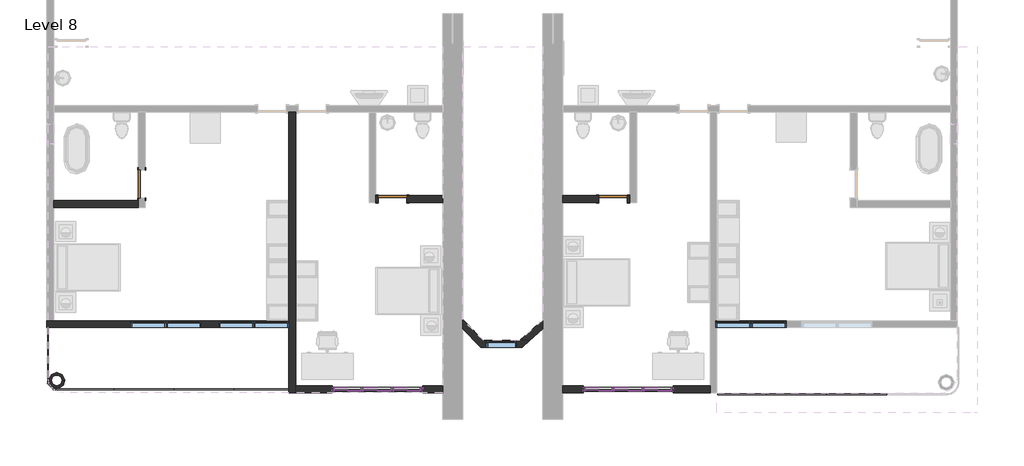
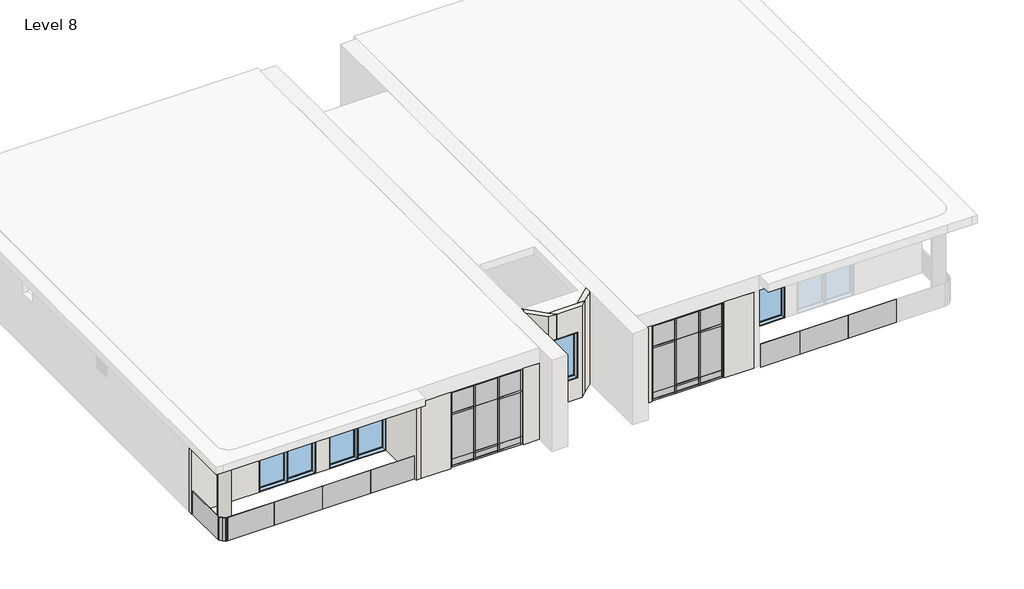
# One storey, part 1 of 3: 42 members, 30 plates, 14 walls, 7 windows, 3 doors.
"""IFC4 building model written with IfcOpenShell, lengths in millimetres."""

from ifc_helpers import new_model, si_unit, point, frame, frame_2d, origin, place, context, project, spatial, polyline, circle_curve, trimmed, segment, composite_curve, outline, extrude, faceted_brep, transform, mapped, element, save
from components import door_2703ae13, door_10fd3a06, member_c17f1be2, member_ad567e07, member_d2e7e466, member_7db1855a, member_75d1e245, member_d60e8053, member_3c3dc66a, member_2fae0574, member_410c6227, member_73c23c35, system_panel_glazed_38d54ecf, system_panel_glazed_fbb6c980, system_panel_glazed_4137532c, system_panel_glazed_6230de04, system_panel_glazed_a79f7f85, system_panel_glazed_9a5ea490, system_panel_glazed_95be5de7, system_panel_glazed_1e00a1c5, system_panel_glazed_ffe51582, system_panel_glazed_8f95e3f6, system_panel_glazed_836907cd, system_panel_glazed_688a65a2, system_panel_glazed_c1a1c740, system_panel_glazed_22bcd51f, window_9a779fa2, window_1a213a25

model = new_model("IFC4")

# Units and contexts
model_context = context("Model", 3, world=origin())
ifc_project = project(units=[si_unit("LENGTHUNIT", "METRE", prefix="MILLI")], contexts=[model_context])

# Site, building, storey
site = spatial("IfcSite", under=ifc_project)
building = spatial("IfcBuilding", under=site)
storey = spatial("IfcBuildingStorey", under=building, Name="Level 8", Elevation=25603.2)

# Doors
placement = place(None, origin())
door_shape = door_2703ae13(model_context)
element("IfcDoor", 1, ObjectType="Door-Single-Panel.0001 : 34\" x 80\"", at=placement, inside=storey, context=model_context, shape_type="MappedRepresentation", body=[
    mapped(door_shape, transform((-15765.9987704, -441.9241442, 25603.2), x_axis=(0.0, -1.0, 0.0), y_axis=(1.0, 0.0, 0.0), z_axis=(0.0, 0.0, 1.0))),
])
element("IfcDoor", 2, ObjectType="Door-Single-Panel.0001 : 34\" x 80\"", at=placement, inside=storey, context=model_context, shape_type="MappedRepresentation", body=[
    mapped(door_shape, transform((-8145.9987704, -899.1241442, 25603.2), x_axis=(-1.0, 0.0, 0.0), y_axis=(0.0, -1.0, 0.0), z_axis=(0.0, 0.0, 1.0))),
])
door_2_shape = door_10fd3a06(model_context)
element("IfcDoor", 3, ObjectType="Door-Single-Panel.0001 : 34\" x 80\"", at=placement, inside=storey, context=model_context, shape_type="MappedRepresentation", body=[
    mapped(door_2_shape, transform((-1440.3987704, -899.1241442, 25603.2), x_axis=(1.0, 0.0, 0.0), y_axis=(0.0, 1.0, 0.0), z_axis=(0.0, 0.0, 1.0))),
])

# Members
member_shape = member_c17f1be2(model_context)
element("IfcMember", 4, ObjectType="Rectangular Mullion : 2.5\" x 5\" rectangular", at=placement, inside=storey, context=model_context, shape_type="MappedRepresentation", body=[
    mapped(member_shape, transform((-9911.2987704, -6690.3241442, 28651.2), x_axis=(0.0, 0.0, 1.0), y_axis=(0.0, 1.0, 0.0), z_axis=(-1.0, 0.0, 0.0))),
])
element("IfcMember", 5, ObjectType="Rectangular Mullion : 2.5\" x 5\" rectangular", at=placement, inside=storey, context=model_context, shape_type="MappedRepresentation", body=[
    mapped(member_shape, transform((-8114.2487704, -6690.3241442, 28651.2), x_axis=(0.0, 0.0, 1.0), y_axis=(0.0, 1.0, 0.0), z_axis=(-1.0, 0.0, 0.0))),
])
element("IfcMember", 6, ObjectType="Rectangular Mullion : 2.5\" x 5\" rectangular", at=placement, inside=storey, context=model_context, shape_type="MappedRepresentation", body=[
    mapped(member_shape, transform((-2291.2987704, -6690.3241442, 28651.2), x_axis=(0.0, 0.0, 1.0), y_axis=(0.0, 1.0, 0.0), z_axis=(-1.0, 0.0, 0.0))),
])
element("IfcMember", 7, ObjectType="Rectangular Mullion : 2.5\" x 5\" rectangular", at=placement, inside=storey, context=model_context, shape_type="MappedRepresentation", body=[
    mapped(member_shape, transform((-494.2487704, -6690.3241442, 28651.2), x_axis=(0.0, 0.0, 1.0), y_axis=(0.0, 1.0, 0.0), z_axis=(-1.0, 0.0, 0.0))),
])
element("IfcMember", 8, ObjectType="Rectangular Mullion : 2.5\" x 5\" rectangular", at=placement, inside=storey, context=model_context, shape_type="MappedRepresentation", body=[
    mapped(member_shape, transform((-7295.0987704, -6690.3241442, 25603.2), x_axis=(0.0, 0.0, -1.0), y_axis=(0.0, 1.0, 0.0), z_axis=(1.0, 0.0, 0.0))),
])
element("IfcMember", 9, ObjectType="Rectangular Mullion : 2.5\" x 5\" rectangular", at=placement, inside=storey, context=model_context, shape_type="MappedRepresentation", body=[
    mapped(member_shape, transform((-9092.1487704, -6690.3241442, 25603.2), x_axis=(0.0, 0.0, -1.0), y_axis=(0.0, 1.0, 0.0), z_axis=(1.0, 0.0, 0.0))),
])
element("IfcMember", 10, ObjectType="Rectangular Mullion : 2.5\" x 5\" rectangular", at=placement, inside=storey, context=model_context, shape_type="MappedRepresentation", body=[
    mapped(member_shape, transform((324.9012296, -6690.3241442, 25603.2), x_axis=(0.0, 0.0, -1.0), y_axis=(0.0, 1.0, 0.0), z_axis=(1.0, 0.0, 0.0))),
])
element("IfcMember", 11, ObjectType="Rectangular Mullion : 2.5\" x 5\" rectangular", at=placement, inside=storey, context=model_context, shape_type="MappedRepresentation", body=[
    mapped(member_shape, transform((-1472.1487704, -6690.3241442, 25603.2), x_axis=(0.0, 0.0, -1.0), y_axis=(0.0, 1.0, 0.0), z_axis=(1.0, 0.0, 0.0))),
])
member_2_shape = member_ad567e07(model_context)
element("IfcMember", 12, ObjectType="Rectangular Mullion : 2.5\" x 5\" rectangular", at=placement, inside=storey, context=model_context, shape_type="MappedRepresentation", body=[
    mapped(member_2_shape, transform((-8114.2487704, -6690.3241442, 27736.8), x_axis=(0.0, 0.0, 1.0), y_axis=(0.0, 1.0, 0.0), z_axis=(-1.0, 0.0, 0.0))),
])
element("IfcMember", 13, ObjectType="Rectangular Mullion : 2.5\" x 5\" rectangular", at=placement, inside=storey, context=model_context, shape_type="MappedRepresentation", body=[
    mapped(member_2_shape, transform((-9911.2987704, -6690.3241442, 27736.8), x_axis=(0.0, 0.0, 1.0), y_axis=(0.0, 1.0, 0.0), z_axis=(-1.0, 0.0, 0.0))),
])
element("IfcMember", 14, ObjectType="Rectangular Mullion : 2.5\" x 5\" rectangular", at=placement, inside=storey, context=model_context, shape_type="MappedRepresentation", body=[
    mapped(member_2_shape, transform((-494.2487704, -6690.3241442, 27736.8), x_axis=(0.0, 0.0, 1.0), y_axis=(0.0, 1.0, 0.0), z_axis=(-1.0, 0.0, 0.0))),
])
element("IfcMember", 15, ObjectType="Rectangular Mullion : 2.5\" x 5\" rectangular", at=placement, inside=storey, context=model_context, shape_type="MappedRepresentation", body=[
    mapped(member_2_shape, transform((-2291.2987704, -6690.3241442, 27736.8), x_axis=(0.0, 0.0, 1.0), y_axis=(0.0, 1.0, 0.0), z_axis=(-1.0, 0.0, 0.0))),
])
member_3_shape = member_d2e7e466(model_context)
element("IfcMember", 16, ObjectType="Rectangular Mullion : 2.5\" x 5\" rectangular", at=placement, inside=storey, context=model_context, shape_type="MappedRepresentation", body=[
    mapped(member_3_shape, transform((-8177.7487704, -6690.3241442, 25603.2), x_axis=(0.0, 0.0, -1.0), y_axis=(0.0, 1.0, 0.0), z_axis=(1.0, 0.0, 0.0))),
])
element("IfcMember", 17, ObjectType="Rectangular Mullion : 2.5\" x 5\" rectangular", at=placement, inside=storey, context=model_context, shape_type="MappedRepresentation", body=[
    mapped(member_3_shape, transform((-557.7487704, -6690.3241442, 25603.2), x_axis=(0.0, 0.0, -1.0), y_axis=(0.0, 1.0, 0.0), z_axis=(1.0, 0.0, 0.0))),
])
member_4_shape = member_7db1855a(model_context)
element("IfcMember", 18, ObjectType="Rectangular Mullion : 2.5\" x 5\" rectangular", at=placement, inside=storey, context=model_context, shape_type="MappedRepresentation", body=[
    mapped(member_4_shape, transform((-9028.6487704, -6690.3241442, 25908.0), x_axis=(0.0, 0.0, 1.0), y_axis=(0.0, 1.0, 0.0), z_axis=(-1.0, 0.0, 0.0))),
])
element("IfcMember", 19, ObjectType="Rectangular Mullion : 2.5\" x 5\" rectangular", at=placement, inside=storey, context=model_context, shape_type="MappedRepresentation", body=[
    mapped(member_4_shape, transform((-1408.6487704, -6690.3241442, 25908.0), x_axis=(0.0, 0.0, 1.0), y_axis=(0.0, 1.0, 0.0), z_axis=(-1.0, 0.0, 0.0))),
])
element("IfcMember", 20, ObjectType="Rectangular Mullion : 2.5\" x 5\" rectangular", at=placement, inside=storey, context=model_context, shape_type="MappedRepresentation", body=[
    mapped(member_3_shape, transform((-9028.6487704, -6690.3241442, 28651.2), x_axis=(0.0, 0.0, 1.0), y_axis=(0.0, 1.0, 0.0), z_axis=(-1.0, 0.0, 0.0))),
])
element("IfcMember", 21, ObjectType="Rectangular Mullion : 2.5\" x 5\" rectangular", at=placement, inside=storey, context=model_context, shape_type="MappedRepresentation", body=[
    mapped(member_3_shape, transform((-1408.6487704, -6690.3241442, 28651.2), x_axis=(0.0, 0.0, 1.0), y_axis=(0.0, 1.0, 0.0), z_axis=(-1.0, 0.0, 0.0))),
])
member_5_shape = member_75d1e245(model_context)
element("IfcMember", 22, ObjectType="Rectangular Mullion : 2.5\" x 5\" rectangular", at=placement, inside=storey, context=model_context, shape_type="MappedRepresentation", body=[
    mapped(member_5_shape, transform((-8145.9987704, -6690.3241442, 25603.2), x_axis=(-1.0, 0.0, 0.0), y_axis=(0.0, 1.0, 0.0), z_axis=(0.0, 0.0, -1.0))),
])
element("IfcMember", 23, ObjectType="Rectangular Mullion : 2.5\" x 5\" rectangular", at=placement, inside=storey, context=model_context, shape_type="MappedRepresentation", body=[
    mapped(member_5_shape, transform((-9060.3987704, -6690.3241442, 25603.2), x_axis=(-1.0, 0.0, 0.0), y_axis=(0.0, 1.0, 0.0), z_axis=(0.0, 0.0, -1.0))),
])
element("IfcMember", 24, ObjectType="Rectangular Mullion : 2.5\" x 5\" rectangular", at=placement, inside=storey, context=model_context, shape_type="MappedRepresentation", body=[
    mapped(member_5_shape, transform((-525.9987704, -6690.3241442, 25603.2), x_axis=(-1.0, 0.0, 0.0), y_axis=(0.0, 1.0, 0.0), z_axis=(0.0, 0.0, -1.0))),
])
element("IfcMember", 25, ObjectType="Rectangular Mullion : 2.5\" x 5\" rectangular", at=placement, inside=storey, context=model_context, shape_type="MappedRepresentation", body=[
    mapped(member_5_shape, transform((-1440.3987704, -6690.3241442, 25603.2), x_axis=(-1.0, 0.0, 0.0), y_axis=(0.0, 1.0, 0.0), z_axis=(0.0, 0.0, -1.0))),
])
member_6_shape = member_d60e8053(model_context)
element("IfcMember", 26, ObjectType="Rectangular Mullion : 2.5\" x 5\" rectangular", at=placement, inside=storey, context=model_context, shape_type="MappedRepresentation", body=[
    mapped(member_6_shape, transform((-8145.9987704, -6690.3241442, 25908.0), x_axis=(-1.0, 0.0, 0.0), y_axis=(0.0, 1.0, 0.0), z_axis=(0.0, 0.0, -1.0))),
])
element("IfcMember", 27, ObjectType="Rectangular Mullion : 2.5\" x 5\" rectangular", at=placement, inside=storey, context=model_context, shape_type="MappedRepresentation", body=[
    mapped(member_6_shape, transform((-9060.3987704, -6690.3241442, 25908.0), x_axis=(-1.0, 0.0, 0.0), y_axis=(0.0, 1.0, 0.0), z_axis=(0.0, 0.0, -1.0))),
])
element("IfcMember", 28, ObjectType="Rectangular Mullion : 2.5\" x 5\" rectangular", at=placement, inside=storey, context=model_context, shape_type="MappedRepresentation", body=[
    mapped(member_6_shape, transform((-525.9987704, -6690.3241442, 25908.0), x_axis=(-1.0, 0.0, 0.0), y_axis=(0.0, 1.0, 0.0), z_axis=(0.0, 0.0, -1.0))),
])
element("IfcMember", 29, ObjectType="Rectangular Mullion : 2.5\" x 5\" rectangular", at=placement, inside=storey, context=model_context, shape_type="MappedRepresentation", body=[
    mapped(member_6_shape, transform((-1440.3987704, -6690.3241442, 25908.0), x_axis=(-1.0, 0.0, 0.0), y_axis=(0.0, 1.0, 0.0), z_axis=(0.0, 0.0, -1.0))),
])
member_7_shape = member_3c3dc66a(model_context)
element("IfcMember", 30, ObjectType="Rectangular Mullion : 2.5\" x 5\" rectangular", at=placement, inside=storey, context=model_context, shape_type="MappedRepresentation", body=[
    mapped(member_7_shape, transform((-9974.7987704, -6690.3241442, 25603.2), x_axis=(-1.0, 0.0, 0.0), y_axis=(0.0, 1.0, 0.0), z_axis=(0.0, 0.0, -1.0))),
])
element("IfcMember", 31, ObjectType="Rectangular Mullion : 2.5\" x 5\" rectangular", at=placement, inside=storey, context=model_context, shape_type="MappedRepresentation", body=[
    mapped(member_7_shape, transform((-2354.7987704, -6690.3241442, 25603.2), x_axis=(-1.0, 0.0, 0.0), y_axis=(0.0, 1.0, 0.0), z_axis=(0.0, 0.0, -1.0))),
])
member_8_shape = member_2fae0574(model_context)
element("IfcMember", 32, ObjectType="Rectangular Mullion : 2.5\" x 5\" rectangular", at=placement, inside=storey, context=model_context, shape_type="MappedRepresentation", body=[
    mapped(member_8_shape, transform((-9974.7987704, -6690.3241442, 25908.0), x_axis=(-1.0, 0.0, 0.0), y_axis=(0.0, 1.0, 0.0), z_axis=(0.0, 0.0, -1.0))),
])
element("IfcMember", 33, ObjectType="Rectangular Mullion : 2.5\" x 5\" rectangular", at=placement, inside=storey, context=model_context, shape_type="MappedRepresentation", body=[
    mapped(member_8_shape, transform((-2354.7987704, -6690.3241442, 25908.0), x_axis=(-1.0, 0.0, 0.0), y_axis=(0.0, 1.0, 0.0), z_axis=(0.0, 0.0, -1.0))),
])
element("IfcMember", 34, ObjectType="Rectangular Mullion : 2.5\" x 5\" rectangular", at=placement, inside=storey, context=model_context, shape_type="MappedRepresentation", body=[
    mapped(member_8_shape, transform((-7231.5987704, -6690.3241442, 27736.8), x_axis=(1.0, 0.0, 0.0), y_axis=(0.0, 1.0, 0.0), z_axis=(0.0, 0.0, 1.0))),
])
element("IfcMember", 35, ObjectType="Rectangular Mullion : 2.5\" x 5\" rectangular", at=placement, inside=storey, context=model_context, shape_type="MappedRepresentation", body=[
    mapped(member_8_shape, transform((388.4012296, -6690.3241442, 27736.8), x_axis=(1.0, 0.0, 0.0), y_axis=(0.0, 1.0, 0.0), z_axis=(0.0, 0.0, 1.0))),
])
element("IfcMember", 36, ObjectType="Rectangular Mullion : 2.5\" x 5\" rectangular", at=placement, inside=storey, context=model_context, shape_type="MappedRepresentation", body=[
    mapped(member_7_shape, transform((-7231.5987704, -6690.3241442, 25908.0), x_axis=(1.0, 0.0, 0.0), y_axis=(0.0, 1.0, 0.0), z_axis=(0.0, 0.0, 1.0))),
])
element("IfcMember", 37, ObjectType="Rectangular Mullion : 2.5\" x 5\" rectangular", at=placement, inside=storey, context=model_context, shape_type="MappedRepresentation", body=[
    mapped(member_7_shape, transform((388.4012296, -6690.3241442, 25908.0), x_axis=(1.0, 0.0, 0.0), y_axis=(0.0, 1.0, 0.0), z_axis=(0.0, 0.0, 1.0))),
])
member_9_shape = member_410c6227(model_context)
element("IfcMember", 38, ObjectType="Rectangular Mullion : 2.5\" x 5\" rectangular", at=placement, inside=storey, context=model_context, shape_type="MappedRepresentation", body=[
    mapped(member_9_shape, transform((-8145.9987704, -6690.3241442, 27736.8), x_axis=(-1.0, 0.0, 0.0), y_axis=(0.0, 1.0, 0.0), z_axis=(0.0, 0.0, -1.0))),
])
element("IfcMember", 39, ObjectType="Rectangular Mullion : 2.5\" x 5\" rectangular", at=placement, inside=storey, context=model_context, shape_type="MappedRepresentation", body=[
    mapped(member_9_shape, transform((-9060.3987704, -6690.3241442, 27736.8), x_axis=(-1.0, 0.0, 0.0), y_axis=(0.0, 1.0, 0.0), z_axis=(0.0, 0.0, -1.0))),
])
element("IfcMember", 40, ObjectType="Rectangular Mullion : 2.5\" x 5\" rectangular", at=placement, inside=storey, context=model_context, shape_type="MappedRepresentation", body=[
    mapped(member_9_shape, transform((-525.9987704, -6690.3241442, 27736.8), x_axis=(-1.0, 0.0, 0.0), y_axis=(0.0, 1.0, 0.0), z_axis=(0.0, 0.0, -1.0))),
])
element("IfcMember", 41, ObjectType="Rectangular Mullion : 2.5\" x 5\" rectangular", at=placement, inside=storey, context=model_context, shape_type="MappedRepresentation", body=[
    mapped(member_9_shape, transform((-1440.3987704, -6690.3241442, 27736.8), x_axis=(-1.0, 0.0, 0.0), y_axis=(0.0, 1.0, 0.0), z_axis=(0.0, 0.0, -1.0))),
])
member_10_shape = member_73c23c35(model_context)
element("IfcMember", 42, ObjectType="Rectangular Mullion : 2.5\" x 5\" rectangular", at=placement, inside=storey, context=model_context, shape_type="MappedRepresentation", body=[
    mapped(member_10_shape, transform((-7231.5987704, -6690.3241442, 28651.2), x_axis=(1.0, 0.0, 0.0), y_axis=(0.0, 1.0, 0.0), z_axis=(0.0, 0.0, 1.0))),
])
element("IfcMember", 43, ObjectType="Rectangular Mullion : 2.5\" x 5\" rectangular", at=placement, inside=storey, context=model_context, shape_type="MappedRepresentation", body=[
    mapped(member_10_shape, transform((388.4012296, -6690.3241442, 28651.2), x_axis=(1.0, 0.0, 0.0), y_axis=(0.0, 1.0, 0.0), z_axis=(0.0, 0.0, 1.0))),
])
element("IfcMember", 44, ObjectType="Rectangular Mullion : 2.5\" x 5\" rectangular", at=placement, inside=storey, context=model_context, shape_type="MappedRepresentation", body=[
    mapped(member_10_shape, transform((-9974.7987704, -6690.3241442, 27736.8), x_axis=(-1.0, 0.0, 0.0), y_axis=(0.0, 1.0, 0.0), z_axis=(0.0, 0.0, -1.0))),
])
element("IfcMember", 45, ObjectType="Rectangular Mullion : 2.5\" x 5\" rectangular", at=placement, inside=storey, context=model_context, shape_type="MappedRepresentation", body=[
    mapped(member_10_shape, transform((-2354.7987704, -6690.3241442, 27736.8), x_axis=(-1.0, 0.0, 0.0), y_axis=(0.0, 1.0, 0.0), z_axis=(0.0, 0.0, -1.0))),
])

# Plates
system_panel_glazed_shape = system_panel_glazed_38d54ecf(model_context)
element("IfcPlate", 46, ObjectType="System Panel : Glazed", at=placement, inside=storey, context=model_context, shape_type="MappedRepresentation", body=[
    mapped(system_panel_glazed_shape, transform((-8603.1987704, -6690.3241442, 25939.75), x_axis=(-1.0, 0.0, 0.0), y_axis=(0.0, -1.0, 0.0), z_axis=(0.0, 0.0, 1.0))),
])
element("IfcPlate", 47, ObjectType="System Panel : Glazed", at=placement, inside=storey, context=model_context, shape_type="MappedRepresentation", body=[
    mapped(system_panel_glazed_shape, transform((-983.1987704, -6690.3241442, 25939.75), x_axis=(-1.0, 0.0, 0.0), y_axis=(0.0, -1.0, 0.0), z_axis=(0.0, 0.0, 1.0))),
])
system_panel_glazed_2_shape = system_panel_glazed_fbb6c980(model_context)
element("IfcPlate", 48, ObjectType="System Panel : Glazed", at=placement, inside=storey, context=model_context, shape_type="MappedRepresentation", body=[
    mapped(system_panel_glazed_2_shape, transform((-8603.1987704, -6690.3241442, 25666.7), x_axis=(-1.0, 0.0, 0.0), y_axis=(0.0, -1.0, 0.0), z_axis=(0.0, 0.0, 1.0))),
])
element("IfcPlate", 49, ObjectType="System Panel : Glazed", at=placement, inside=storey, context=model_context, shape_type="MappedRepresentation", body=[
    mapped(system_panel_glazed_2_shape, transform((-983.1987704, -6690.3241442, 25666.7), x_axis=(-1.0, 0.0, 0.0), y_axis=(0.0, -1.0, 0.0), z_axis=(0.0, 0.0, 1.0))),
])
system_panel_glazed_3_shape = system_panel_glazed_4137532c(model_context)
element("IfcPlate", 50, ObjectType="System Panel : Glazed", at=placement, inside=storey, context=model_context, shape_type="MappedRepresentation", body=[
    mapped(system_panel_glazed_3_shape, transform((-7704.6737704, -6690.3241442, 25666.7), x_axis=(-1.0, 0.0, 0.0), y_axis=(0.0, -1.0, 0.0), z_axis=(0.0, 0.0, 1.0))),
])
element("IfcPlate", 51, ObjectType="System Panel : Glazed", at=placement, inside=storey, context=model_context, shape_type="MappedRepresentation", body=[
    mapped(system_panel_glazed_3_shape, transform((-9501.7237704, -6690.3241442, 25666.7), x_axis=(-1.0, 0.0, 0.0), y_axis=(0.0, -1.0, 0.0), z_axis=(0.0, 0.0, 1.0))),
])
element("IfcPlate", 52, ObjectType="System Panel : Glazed", at=placement, inside=storey, context=model_context, shape_type="MappedRepresentation", body=[
    mapped(system_panel_glazed_3_shape, transform((-84.6737704, -6690.3241442, 25666.7), x_axis=(-1.0, 0.0, 0.0), y_axis=(0.0, -1.0, 0.0), z_axis=(0.0, 0.0, 1.0))),
])
element("IfcPlate", 53, ObjectType="System Panel : Glazed", at=placement, inside=storey, context=model_context, shape_type="MappedRepresentation", body=[
    mapped(system_panel_glazed_3_shape, transform((-1881.7237704, -6690.3241442, 25666.7), x_axis=(-1.0, 0.0, 0.0), y_axis=(0.0, -1.0, 0.0), z_axis=(0.0, 0.0, 1.0))),
])
system_panel_glazed_4_shape = system_panel_glazed_6230de04(model_context)
element("IfcPlate", 54, ObjectType="System Panel : Glazed", at=placement, inside=storey, context=model_context, shape_type="MappedRepresentation", body=[
    mapped(system_panel_glazed_4_shape, transform((-7704.6737704, -6690.3241442, 25908.0), x_axis=(-1.0, 0.0, 0.0), y_axis=(0.0, -1.0, 0.0), z_axis=(0.0, 0.0, 1.0))),
])
element("IfcPlate", 55, ObjectType="System Panel : Glazed", at=placement, inside=storey, context=model_context, shape_type="MappedRepresentation", body=[
    mapped(system_panel_glazed_4_shape, transform((-9501.7237704, -6690.3241442, 25908.0), x_axis=(-1.0, 0.0, 0.0), y_axis=(0.0, -1.0, 0.0), z_axis=(0.0, 0.0, 1.0))),
])
element("IfcPlate", 56, ObjectType="System Panel : Glazed", at=placement, inside=storey, context=model_context, shape_type="MappedRepresentation", body=[
    mapped(system_panel_glazed_4_shape, transform((-84.6737704, -6690.3241442, 25908.0), x_axis=(-1.0, 0.0, 0.0), y_axis=(0.0, -1.0, 0.0), z_axis=(0.0, 0.0, 1.0))),
])
element("IfcPlate", 57, ObjectType="System Panel : Glazed", at=placement, inside=storey, context=model_context, shape_type="MappedRepresentation", body=[
    mapped(system_panel_glazed_4_shape, transform((-1881.7237704, -6690.3241442, 25908.0), x_axis=(-1.0, 0.0, 0.0), y_axis=(0.0, -1.0, 0.0), z_axis=(0.0, 0.0, 1.0))),
])
system_panel_glazed_5_shape = system_panel_glazed_a79f7f85(model_context)
element("IfcPlate", 58, ObjectType="System Panel : Glazed", at=placement, inside=storey, context=model_context, shape_type="MappedRepresentation", body=[
    mapped(system_panel_glazed_5_shape, transform((-7704.6737704, -6690.3241442, 27768.55), x_axis=(-1.0, 0.0, 0.0), y_axis=(0.0, -1.0, 0.0), z_axis=(0.0, 0.0, 1.0))),
])
element("IfcPlate", 59, ObjectType="System Panel : Glazed", at=placement, inside=storey, context=model_context, shape_type="MappedRepresentation", body=[
    mapped(system_panel_glazed_5_shape, transform((-9501.7237704, -6690.3241442, 27768.55), x_axis=(-1.0, 0.0, 0.0), y_axis=(0.0, -1.0, 0.0), z_axis=(0.0, 0.0, 1.0))),
])
element("IfcPlate", 60, ObjectType="System Panel : Glazed", at=placement, inside=storey, context=model_context, shape_type="MappedRepresentation", body=[
    mapped(system_panel_glazed_5_shape, transform((-84.6737704, -6690.3241442, 27768.55), x_axis=(-1.0, 0.0, 0.0), y_axis=(0.0, -1.0, 0.0), z_axis=(0.0, 0.0, 1.0))),
])
element("IfcPlate", 61, ObjectType="System Panel : Glazed", at=placement, inside=storey, context=model_context, shape_type="MappedRepresentation", body=[
    mapped(system_panel_glazed_5_shape, transform((-1881.7237704, -6690.3241442, 27768.55), x_axis=(-1.0, 0.0, 0.0), y_axis=(0.0, -1.0, 0.0), z_axis=(0.0, 0.0, 1.0))),
])
system_panel_glazed_6_shape = system_panel_glazed_9a5ea490(model_context)
element("IfcPlate", 62, ObjectType="System Panel : Glazed", at=placement, inside=storey, context=model_context, shape_type="MappedRepresentation", body=[
    mapped(system_panel_glazed_6_shape, transform((-8603.1987704, -6690.3241442, 27736.8), x_axis=(-1.0, 0.0, 0.0), y_axis=(0.0, -1.0, 0.0), z_axis=(0.0, 0.0, 1.0))),
])
element("IfcPlate", 63, ObjectType="System Panel : Glazed", at=placement, inside=storey, context=model_context, shape_type="MappedRepresentation", body=[
    mapped(system_panel_glazed_6_shape, transform((-983.1987704, -6690.3241442, 27736.8), x_axis=(-1.0, 0.0, 0.0), y_axis=(0.0, -1.0, 0.0), z_axis=(0.0, 0.0, 1.0))),
])
system_panel_glazed_7_shape = system_panel_glazed_95be5de7(model_context)
element("IfcPlate", 64, ObjectType="System Panel : Glazed", at=placement, inside=storey, context=model_context, shape_type="MappedRepresentation", body=[
    mapped(system_panel_glazed_7_shape, transform((-15707.2305745, -6723.6923401, 25603.2), x_axis=(1.0, 0.0, 0.0), y_axis=(0.0, 1.0, 0.0), z_axis=(0.0, 0.0, 1.0))),
])
element("IfcPlate", 65, ObjectType="System Panel : Glazed", at=placement, inside=storey, context=model_context, shape_type="MappedRepresentation", body=[
    mapped(system_panel_glazed_7_shape, transform((-13878.4305745, -6723.6923401, 25603.2), x_axis=(1.0, 0.0, 0.0), y_axis=(0.0, 1.0, 0.0), z_axis=(0.0, 0.0, 1.0))),
])
element("IfcPlate", 66, ObjectType="System Panel : Glazed", at=placement, inside=storey, context=model_context, shape_type="MappedRepresentation", body=[
    mapped(system_panel_glazed_7_shape, transform((5957.9120092, -6810.4133646, 25603.2), x_axis=(-1.0, 0.0, 0.0), y_axis=(0.0, -1.0, 0.0), z_axis=(0.0, 0.0, 1.0))),
])
element("IfcPlate", 67, ObjectType="System Panel : Glazed", at=placement, inside=storey, context=model_context, shape_type="MappedRepresentation", body=[
    mapped(system_panel_glazed_7_shape, transform((4129.1120092, -6810.4133646, 25603.2), x_axis=(-1.0, 0.0, 0.0), y_axis=(0.0, -1.0, 0.0), z_axis=(0.0, 0.0, 1.0))),
])
system_panel_glazed_8_shape = system_panel_glazed_1e00a1c5(model_context)
element("IfcPlate", 68, ObjectType="System Panel : Glazed", at=placement, inside=storey, context=model_context, shape_type="MappedRepresentation", body=[
    mapped(system_panel_glazed_8_shape, transform((2478.1120092, -6810.4133646, 25603.2), x_axis=(-1.0, 0.0, 0.0), y_axis=(0.0, -1.0, 0.0), z_axis=(0.0, 0.0, 1.0))),
])
system_panel_glazed_9_shape = system_panel_glazed_ffe51582(model_context)
element("IfcPlate", 69, ObjectType="System Panel : Glazed", at=placement, inside=storey, context=model_context, shape_type="MappedRepresentation", body=[
    mapped(system_panel_glazed_9_shape, transform((-18451.9713429, -6722.1515718, 25603.2), x_axis=(0.7071067811865462, -0.7071067811865488, 0.0), y_axis=(0.7071067811865488, 0.7071067811865462, 0.0), z_axis=(0.0, 0.0, 1.0))),
])
system_panel_glazed_10_shape = system_panel_glazed_8f95e3f6(model_context)
element("IfcPlate", 70, ObjectType="System Panel : Glazed", at=placement, inside=storey, context=model_context, shape_type="MappedRepresentation", body=[
    mapped(system_panel_glazed_10_shape, transform((-18648.8987704, -5667.9741442, 25603.2), x_axis=(0.0, -1.0, 0.0), y_axis=(1.0, 0.0, 0.0), z_axis=(0.0, 0.0, 1.0))),
])
system_panel_glazed_11_shape = system_panel_glazed_836907cd(model_context)
element("IfcPlate", 71, ObjectType="System Panel : Glazed", at=placement, inside=storey, context=model_context, shape_type="MappedRepresentation", body=[
    mapped(system_panel_glazed_11_shape, transform((-18418.6805745, -6723.6923401, 25603.2), x_axis=(1.0, 0.0, 0.0), y_axis=(0.0, 1.0, 0.0), z_axis=(0.0, 0.0, 1.0))),
])
system_panel_glazed_12_shape = system_panel_glazed_688a65a2(model_context)
element("IfcPlate", 72, ObjectType="System Panel : Glazed", at=placement, inside=storey, context=model_context, shape_type="MappedRepresentation", body=[
    mapped(system_panel_glazed_12_shape, transform((-12129.8146725, -6723.6923401, 25603.2), x_axis=(1.0, 0.0, 0.0), y_axis=(0.0, 1.0, 0.0), z_axis=(0.0, 0.0, 1.0))),
])
system_panel_glazed_13_shape = system_panel_glazed_c1a1c740(model_context)
element("IfcPlate", 73, ObjectType="System Panel : Glazed", at=placement, inside=storey, context=model_context, shape_type="MappedRepresentation", body=[
    mapped(system_panel_glazed_13_shape, transform((-17504.2805745, -6723.6923401, 25603.2), x_axis=(1.0, 0.0, 0.0), y_axis=(0.0, 1.0, 0.0), z_axis=(0.0, 0.0, 1.0))),
])
system_panel_glazed_14_shape = system_panel_glazed_22bcd51f(model_context)
element("IfcPlate", 74, ObjectType="System Panel : Glazed", at=placement, inside=storey, context=model_context, shape_type="MappedRepresentation", body=[
    mapped(system_panel_glazed_14_shape, transform((-18600.0521056, -6574.070809, 25603.2), x_axis=(0.7071067811865462, -0.7071067811865488, 0.0), y_axis=(0.7071067811865488, 0.7071067811865462, 0.0), z_axis=(0.0, 0.0, 1.0))),
])
element("IfcPlate", 75, ObjectType="System Panel : Glazed", at=placement, inside=storey, context=model_context, shape_type="MappedRepresentation", body=[
    mapped(system_panel_glazed_14_shape, transform((-18502.3587761, -6671.7641386, 25603.2), x_axis=(0.7071067811865462, -0.7071067811865488, 0.0), y_axis=(0.7071067811865488, 0.7071067811865462, 0.0), z_axis=(0.0, 0.0, 1.0))),
])

# Walls
element("IfcWall", 76, ObjectType="Generic - 3\" green 2", at=placement, inside=storey, context=model_context, shape_type="SweptSolid", body=[
    extrude(outline(composite_curve([segment(polyline([(-18518.7237704, -6418.8616442), (-18594.9237704, -6418.8616442)]), True, "CONTINUOUS"), segment(trimmed(circle_curve(frame_2d((-18353.6237704, -6418.8616442)), 241.3), [point((-18594.9237704, -6418.8616442))], [point((-18112.3237704, -6418.8616442))], False, "CARTESIAN"), True, "CONTINUOUS"), segment(polyline([(-18112.3237704, -6418.8616442), (-18188.5237704, -6418.8616442)]), True, "CONTINUOUS"), segment(trimmed(circle_curve(frame_2d((-18353.6237704, -6418.8616442)), 165.1), [point((-18188.5237704, -6418.8616442))], [point((-18518.7237704, -6418.8616442))], True, "CARTESIAN"), True, "CONTINUOUS")], self_intersect=False)), frame((0.0, 0.0, 25603.2), z_axis=(0.0, 0.0, 1.0), x_axis=(1.0, 0.0, 0.0)), (0.0, 0.0, 1.0), 3048.0),
])
element("IfcWall", 77, ObjectType="Generic - 3\" green 2", at=placement, inside=storey, context=model_context, shape_type="SweptSolid", body=[
    extrude(outline(composite_curve([segment(polyline([(-18188.5237704, -6418.8616442), (-18112.3237704, -6418.8616442)]), True, "CONTINUOUS"), segment(trimmed(circle_curve(frame_2d((-18353.6237704, -6418.8616442)), 241.3), [point((-18112.3237704, -6418.8616442))], [point((-18594.9237704, -6418.8616442))], False, "CARTESIAN"), True, "CONTINUOUS"), segment(polyline([(-18594.9237704, -6418.8616442), (-18518.7237704, -6418.8616442)]), True, "CONTINUOUS"), segment(trimmed(circle_curve(frame_2d((-18353.6237704, -6418.8616442)), 165.1), [point((-18518.7237704, -6418.8616442))], [point((-18188.5237704, -6418.8616442))], True, "CARTESIAN"), True, "CONTINUOUS")], self_intersect=False)), frame((0.0, 0.0, 25603.2), z_axis=(0.0, 0.0, 1.0), x_axis=(1.0, 0.0, 0.0)), (0.0, 0.0, 1.0), 3048.0),
])
element("IfcWall", 78, ObjectType="Generic - 8\" cream", at=placement, inside=storey, context=model_context, shape_type="Brep", body=[
    faceted_brep([(-11295.5987704, 1742.4758558, 25603.2), (-11295.5987704, -6791.9241442, 25603.2), (-11295.5987704, -6791.9241442, 28651.2), (-11295.5987704, -4810.7241442, 28651.2), (-11295.5987704, -4607.5241442, 28651.2), (-11295.5987704, 1742.4758558, 28651.2), (-11092.3987704, 1742.4758558, 25603.2), (-11092.3987704, 1742.4758558, 28651.2), (-11092.3987704, -6588.7241442, 28651.2), (-11092.3987704, -6791.9241442, 28651.2), (-11092.3987704, -6791.9241442, 25603.2), (-11092.3987704, -6588.7241442, 25603.2)], [[[0, 1, 2, 3, 4, 5]], [[6, 7, 8, 9, 10, 11]], [[1, 0, 6, 11, 10]], [[5, 4, 3, 2, 9, 8, 7]], [[0, 5, 7, 6]], [[2, 1, 10, 9]]]),
])
element("IfcWall", 79, ObjectType="Generic - 8\" cream", at=placement, inside=storey, context=model_context, shape_type="SweptSolid", body=[
    extrude(outline(polyline([(-18445.6987704, -949.9241442), (-15867.5987704, -949.9241442), (-15867.5987704, -1153.1241442), (-18445.6987704, -1153.1241442), (-18445.6987704, -949.9241442)])), frame((0.0, 0.0, 25603.2), z_axis=(0.0, 0.0, 1.0), x_axis=(1.0, 0.0, 0.0)), (0.0, 0.0, 1.0), 3048.0),
])
element("IfcWall", 80, ObjectType="Generic - 8\" cream", at=placement, inside=storey, context=model_context, shape_type="SweptSolid", body=[
    extrude(outline(polyline([(28651.2, -6621.9987704), (28651.2, -8653.9987704), (25603.2, -8653.9987704), (25603.2, -8577.7987704), (27635.2, -8577.7987704), (27635.2, -7714.1987704), (25603.2, -7714.1987704), (25603.2, -6621.9987704), (28651.2, -6621.9987704)])), frame((0.0, -1000.7241442, 0.0), z_axis=(0.0, 1.0, 0.0), x_axis=(0.0, 0.0, 1.0)), (0.0, 0.0, 1.0), 203.2),
])
element("IfcWall", 81, ObjectType="Generic - 8\" cream", at=placement, inside=storey, context=model_context, shape_type="Brep", body=[
    faceted_brep([(-18648.8987704, -4607.5241442, 28651.2), (-18445.6987704, -4607.5241442, 28651.2), (-11295.5987704, -4607.5241442, 28651.2), (-11295.5987704, -4607.5241442, 28346.4), (-13429.1987704, -4607.5241442, 28346.4), (-13429.1987704, -4607.5241442, 25603.2), (-13962.5987704, -4607.5241442, 25603.2), (-13962.5987704, -4607.5241442, 28346.4), (-16096.1987704, -4607.5241442, 28346.4), (-16096.1987704, -4607.5241442, 25603.2), (-18445.6987704, -4607.5241442, 25603.2), (-18648.8987704, -4607.5241442, 25603.2), (-11295.5987704, -4810.7241442, 28651.2), (-18648.8987704, -4810.7241442, 28651.2), (-18648.8987704, -4810.7241442, 25603.2), (-16096.1987704, -4810.7241442, 25603.2), (-16096.1987704, -4810.7241442, 28346.4), (-13962.5987704, -4810.7241442, 28346.4), (-13962.5987704, -4810.7241442, 25603.2), (-13429.1987704, -4810.7241442, 25603.2), (-13429.1987704, -4810.7241442, 28346.4), (-11295.5987704, -4810.7241442, 28346.4)], [[[0, 1, 2, 3, 4, 5, 6, 7, 8, 9, 10, 11]], [[12, 13, 14, 15, 16, 17, 18, 19, 20, 21]], [[14, 11, 10, 9, 15]], [[5, 19, 18, 6]], [[2, 1, 0, 13, 12]], [[2, 12, 21, 3]], [[0, 11, 14, 13]], [[3, 21, 20, 4]], [[4, 20, 19, 5]], [[17, 7, 6, 18]], [[7, 17, 16, 8]], [[8, 16, 15, 9]]]),
])
element("IfcWall", 82, ObjectType="Generic - 8\" cream", at=placement, inside=storey, context=model_context, shape_type="SweptSolid", body=[
    extrude(outline(polyline([(28651.2, -932.3987704), (28651.2, -2964.3987704), (25603.2, -2964.3987704), (25603.2, -1872.1987704), (27635.2, -1872.1987704), (27635.2, -1008.5987704), (25603.2, -1008.5987704), (25603.2, -932.3987704), (28651.2, -932.3987704)])), frame((0.0, -1000.7241442, 0.0), z_axis=(0.0, 1.0, 0.0), x_axis=(0.0, 0.0, 1.0)), (0.0, 0.0, 1.0), 203.2),
])
element("IfcWall", 83, ObjectType="Generic - 8\" cream", at=placement, inside=storey, context=model_context, shape_type="SweptSolid", body=[
    extrude(outline(polyline([(388.4012296, -6588.7241442), (1506.0012296, -6588.7241442), (1506.0012296, -6791.9241442), (388.4012296, -6791.9241442), (388.4012296, -6588.7241442)])), frame((0.0, 0.0, 25603.2), z_axis=(0.0, 0.0, 1.0), x_axis=(1.0, 0.0, 0.0)), (0.0, 0.0, 1.0), 3048.0),
])
element("IfcWall", 84, ObjectType="Generic - 8\" cream", at=placement, inside=storey, context=model_context, shape_type="SweptSolid", body=[
    extrude(outline(polyline([(-2354.7987704, -6791.9241442), (-2964.3987704, -6791.9241442), (-2964.3987704, -6588.7241442), (-2354.7987704, -6588.7241442), (-2354.7987704, -6791.9241442)])), frame((0.0, 0.0, 25603.2), z_axis=(0.0, 0.0, 1.0), x_axis=(1.0, 0.0, 0.0)), (0.0, 0.0, 1.0), 3048.0),
])
element("IfcWall", 85, ObjectType="Generic - 8\" cream", at=placement, inside=storey, context=model_context, shape_type="SweptSolid", body=[
    extrude(outline(polyline([(-9974.7987704, -6791.9241442), (-11092.3987704, -6791.9241442), (-11092.3987704, -6588.7241442), (-9974.7987704, -6588.7241442), (-9974.7987704, -6791.9241442)])), frame((0.0, 0.0, 25603.2), z_axis=(0.0, 0.0, 1.0), x_axis=(1.0, 0.0, 0.0)), (0.0, 0.0, 1.0), 3048.0),
])
element("IfcWall", 86, ObjectType="Generic - 8\" cream", at=placement, inside=storey, context=model_context, shape_type="SweptSolid", body=[
    extrude(outline(polyline([(-7231.5987704, -6588.7241442), (-6621.9987704, -6588.7241442), (-6621.9987704, -6791.9241442), (-7231.5987704, -6791.9241442), (-7231.5987704, -6588.7241442)])), frame((0.0, 0.0, 25603.2), z_axis=(0.0, 0.0, 1.0), x_axis=(1.0, 0.0, 0.0)), (0.0, 0.0, 1.0), 3048.0),
])
element("IfcWall", 87, ObjectType="Generic - 8\" green", at=placement, inside=storey, context=model_context, shape_type="Brep", body=[
    faceted_brep([(-6012.3987704, -4852.8082422, 25603.2), (-5458.7044276, -5406.502585, 25603.2), (-5458.7044276, -5406.502585, 29260.8), (-6012.3987704, -4852.8082422, 29260.8), (-5171.3362318, -5406.502585, 25603.2), (-5374.5362318, -5203.302585, 25603.2), (-6012.3987704, -4565.4400463, 25603.2), (-6012.3987704, -4565.4400463, 29260.8), (-5374.5362318, -5203.302585, 29260.8), (-5171.3362318, -5406.502585, 29260.8), (-5171.3362318, -5406.502585, 28270.2), (-5289.4901401, -5288.3486766, 28270.2), (-5289.4901401, -5288.3486766, 26441.4), (-5171.3362318, -5406.502585, 26441.4), (-5289.4901401, -5406.502585, 26441.4), (-5289.4901401, -5406.502585, 28270.2)], [[[0, 1, 2, 3]], [[4, 5, 6, 7, 8, 9, 10, 11, 12, 13]], [[1, 0, 6, 5, 4]], [[3, 2, 9, 8, 7]], [[0, 3, 7, 6]], [[2, 1, 4, 13, 14, 15, 10, 9]], [[12, 14, 13]], [[14, 12, 11, 15]], [[15, 11, 10]]]),
])
element("IfcWall", 88, ObjectType="Generic - 8\" green", at=placement, inside=storey, context=model_context, shape_type="Brep", body=[
    faceted_brep([(-5171.3362318, -5406.502585, 25603.2), (-4203.3343712, -5406.502585, 25603.2), (-4203.3343712, -5406.502585, 29260.8), (-5171.3362318, -5406.502585, 29260.8), (-5171.3362318, -5406.502585, 28270.2), (-4375.0901401, -5406.502585, 28270.2), (-4375.0901401, -5406.502585, 26441.4), (-5171.3362318, -5406.502585, 26441.4), (-3975.4820774, -5203.302585, 25603.2), (-4280.7801413, -5203.302585, 25603.2), (-5374.5362318, -5203.302585, 25603.2), (-5374.5362318, -5203.302585, 29260.8), (-4280.7801413, -5203.302585, 29260.8), (-3975.4820774, -5203.302585, 29260.8), (-4375.0901401, -5203.302585, 26441.4), (-4375.0901401, -5203.302585, 28270.2), (-5289.4901401, -5203.302585, 28270.2), (-5289.4901401, -5203.302585, 26441.4), (-5289.4901401, -5288.3486766, 26441.4), (-5289.4901401, -5288.3486766, 28270.2)], [[[0, 1, 2, 3, 4, 5, 6, 7]], [[8, 9, 10, 11, 12, 13], [14, 15, 16, 17]], [[1, 0, 10, 9, 8]], [[3, 2, 13, 12, 11]], [[3, 11, 10, 0, 7, 18, 19, 4]], [[2, 1, 8, 13]], [[5, 15, 14, 6]], [[6, 14, 17, 18, 7]], [[18, 17, 16, 19]], [[15, 5, 4, 19, 16]]]),
])
element("IfcWall", 89, ObjectType="Generic - 8\" green", at=placement, inside=storey, context=model_context, shape_type="SweptSolid", body=[
    extrude(outline(polyline([(-3573.9987704, -4845.2574382), (-3975.4820774, -5203.302585), (-4280.7801413, -5203.302585), (-3573.9987704, -4572.9908503), (-3573.9987704, -4845.2574382)])), frame((0.0, 0.0, 25603.2), z_axis=(0.0, 0.0, 1.0), x_axis=(1.0, 0.0, 0.0)), (0.0, 0.0, 1.0), 3657.6),
])

# Windows
window_shape = window_9a779fa2(model_context)
element("IfcWindow", 90, ObjectType="Fixed : 36\" x 72\"", at=placement, inside=storey, context=model_context, shape_type="MappedRepresentation", body=[
    mapped(window_shape, transform((-4794.1901401, -5304.902585, 26136.6), x_axis=(1.0, 0.0, 0.0), y_axis=(0.0, 1.0, 0.0), z_axis=(0.0, 0.0, 1.0))),
])
window_2_shape = window_1a213a25(model_context)
element("IfcWindow", 91, ObjectType="Fixed : 36\" x 72\" 2", at=placement, inside=storey, context=model_context, shape_type="MappedRepresentation", body=[
    mapped(window_2_shape, transform((-11790.8987704, -4709.1241442, 25298.4), x_axis=(1.0, 0.0, 0.0), y_axis=(0.0, 1.0, 0.0), z_axis=(0.0, 0.0, 1.0))),
])
element("IfcWindow", 92, ObjectType="Fixed : 36\" x 72\" 2", at=placement, inside=storey, context=model_context, shape_type="MappedRepresentation", body=[
    mapped(window_2_shape, transform((-12857.6987704, -4709.1241442, 25298.4), x_axis=(1.0, 0.0, 0.0), y_axis=(0.0, 1.0, 0.0), z_axis=(0.0, 0.0, 1.0))),
])
element("IfcWindow", 93, ObjectType="Fixed : 36\" x 72\" 2", at=placement, inside=storey, context=model_context, shape_type="MappedRepresentation", body=[
    mapped(window_2_shape, transform((-14457.8987704, -4709.1241442, 25298.4), x_axis=(1.0, 0.0, 0.0), y_axis=(0.0, 1.0, 0.0), z_axis=(0.0, 0.0, 1.0))),
])
element("IfcWindow", 94, ObjectType="Fixed : 36\" x 72\" 2", at=placement, inside=storey, context=model_context, shape_type="MappedRepresentation", body=[
    mapped(window_2_shape, transform((-15524.6987704, -4709.1241442, 25298.4), x_axis=(1.0, 0.0, 0.0), y_axis=(0.0, 1.0, 0.0), z_axis=(0.0, 0.0, 1.0))),
])
element("IfcWindow", 95, ObjectType="Fixed : 36\" x 72\" 2", at=placement, inside=storey, context=model_context, shape_type="MappedRepresentation", body=[
    mapped(window_2_shape, transform((2255.3012296, -4709.1241442, 25298.4), x_axis=(1.0, 0.0, 0.0), y_axis=(0.0, 1.0, 0.0), z_axis=(0.0, 0.0, 1.0))),
])
element("IfcWindow", 96, ObjectType="Fixed : 36\" x 72\" 2", at=placement, inside=storey, context=model_context, shape_type="MappedRepresentation", body=[
    mapped(window_2_shape, transform((3331.6262296, -4709.1241442, 25298.4), x_axis=(1.0, 0.0, 0.0), y_axis=(0.0, 1.0, 0.0), z_axis=(0.0, 0.0, 1.0))),
])

save(model, "model.ifc")

# Revit data of these elements
# Type "Door-Single-Panel.0001 : 34\" x 80\""
#   Type Mark = "9"
#   Construction Type Id = "DOOR"
#   Assembly Code = "C1020300"
#   Analytic Construction = "Wooden"
#   Thickness = 0' - 2"
#   Thermal Resistance (R) = 0.455703 (m²·K)/W
#   Swing Angle [instance default] = 90.00°
#   Heat Transfer Coefficient (U) = 2.19465 W/(m²·K)
#   Height = 6' - 8"
#   Trim Projection Ext = 0' - 1"
#   Trim Projection Int = 0' - 1"
#   Trim Width = 0' - 3"
#   Width = 2' - 10"
#   Panel Material = Wood - Birch - Solid Stained Light Low Gloss
#   Trim Material = Paint - Sienna
#   Visual Light Transmittance = 0
#   Solar Heat Gain Coefficient = 0
#   Function = (empty or 0)
#   Wall Closure = (empty or 0)
# Type "Rectangular Mullion : 2.5\" x 5\" rectangular"
#   built-in parameter 1007304 = 0.416667 (stored number, unit not read)
#   built-in parameter 1007301 = 0.104167 (stored number, unit not read)
#   built-in parameter 1007300 = 0.104167 (stored number, unit not read)
# Type "System Panel : Glazed"
#   Construction Type Id = "GSP4R"
#   Analytic Construction = "1/8 in Pilkington single glazing"
#   Visual Light Transmittance = 0.9
#   Solar Heat Gain Coefficient = 0.86
#   Heat Transfer Coefficient (U) = 6.7069 W/(m²·K)
# Type "Generic - 3\" green 2"
#   Assembly Code = "B2010"
#   Width = 0' - 3"
#   Layers, outside or top first: 0' - 3" "Damp-proofing" (function 1)
# Type "Generic - 8\" cream"
#   Assembly Code = "B2010"
#   Width = 0' - 8"
#   Layers, outside or top first: 0' - 8" "Parking Stripe" (function 1)
# Type "Generic - 8\" green"
#   Assembly Code = "B2010"
#   Width = 0' - 8"
#   Layers, outside or top first: 0' - 8" "Damp-proofing" (function 1)
# Type "Fixed : 36\" x 72\""
#   Type Mark = "9"
#   Construction Type Id = "GSP4R"
#   Assembly Code = "B2020100"
#   Analytic Construction = "1/8 in Pilkington single glazing"
#   Visual Light Transmittance = 0.9
#   Solar Heat Gain Coefficient = 0.78
#   Heat Transfer Coefficient (U) = 3.6886 W/(m²·K)
#   Height = 6' - 0"
#   Default Sill Height = 1' - 0"
#   Width = 3' - 0"
#   Window Inset = 0' - 0 3/4"
#   Glass Pane Material = Glass
#   Sash Material = Iron, Ductile
#   Wall Closure = (empty or 0)
# Type "Fixed : 36\" x 72\" 2"
#   Type Mark = "29"
#   Construction Type Id = "GSP4R"
#   Assembly Code = "B2020100"
#   Analytic Construction = "1/8 in Pilkington single glazing"
#   Visual Light Transmittance = 0.9
#   Solar Heat Gain Coefficient = 0.78
#   Heat Transfer Coefficient (U) = 3.6886 W/(m²·K)
#   Height = 9' - 0"
#   Default Sill Height = 1' - 0"
#   Width = 3' - 6"
#   Window Inset = 0' - 0 3/4"
#   Glass Pane Material = Glass
#   Sash Material = Iron, Ductile
#   Wall Closure = (empty or 0)
# Elements 1, 2, 3 (IfcDoor, "Door-Single-Panel.0001 : 34\" x 80\"")
#   Swing Angle = 90.00°
#   Phase Created = New Construction
#   Materials on its faces: "Paint - Sienna", "Wood - Birch - Solid Stained Light Low Gloss"
# Elements 4, 5, 6, 7, 8, 9, 10, 11, 12, 13, 14, 15, 16, 17, 18, 19, 20, 21, 22, 23, 24, 25, 26, 27, 28, 29, 30, 31, 32, 33, 34, 35, 36, 37, 38, 39, 40, 41, 42, 43, 44, 45 (IfcMember, "Rectangular Mullion : 2.5\" x 5\" rectangular")
#   Phase Created = New Construction
#   Materials on its faces: "Iron, Ductile"
# Elements 46, 47, 48, 49, 50, 51, 52, 53, 54, 55, 56, 57, 58, 59, 60, 61, 62, 63, 64, 65, 66, 67, 68, 69, 70, 71, 72, 73, 74, 75 (IfcPlate, "System Panel : Glazed")
#   Phase Created = New Construction
#   Materials on its faces: "Glass"
# Elements 76, 77 (IfcWall, "Generic - 3\" green 2")
#   Top Offset = 0' - 0"
#   Base Offset = 0' - 0"
#   Unconnected Height = 10' - 0"
#   wall height = 10' - 0"
#   Phase Created = New Construction
#   Materials on its faces: "Damp-proofing"
# Elements 78, 79, 80, 81, 82, 83, 84, 85, 86 (IfcWall, "Generic - 8\" cream")
#   Top Offset = 0' - 0"
#   Base Offset = 0' - 0"
#   Unconnected Height = 10' - 0"
#   wall height = 10' - 0"
#   Phase Created = New Construction
#   Base Constraint = Level 8
#   Materials on its faces: "Parking Stripe"
# Elements 87, 88, 89 (IfcWall, "Generic - 8\" green")
#   Top Offset = 0' - 0"
#   Base Offset = 0' - 0"
#   Unconnected Height = 12' - 0"
#   wall height = 12' - 0"
#   Phase Created = New Construction
#   Base Constraint = Level 8
#   Materials on its faces: "Damp-proofing"
# Element 90 (IfcWindow, "Fixed : 36\" x 72\"")
#   Mark = "188"
#   Phase Created = New Construction
#   Materials on its faces: "Iron, Ductile", "Glass"
# Element 91 (IfcWindow, "Fixed : 36\" x 72\" 2")
#   Mark = "189"
#   Phase Created = New Construction
#   Materials on its faces: "Iron, Ductile", "Glass"
# Element 92 (IfcWindow, "Fixed : 36\" x 72\" 2")
#   Mark = "190"
#   Phase Created = New Construction
#   Materials on its faces: "Iron, Ductile", "Glass"
# Element 93 (IfcWindow, "Fixed : 36\" x 72\" 2")
#   Mark = "191"
#   Phase Created = New Construction
#   Materials on its faces: "Iron, Ductile", "Glass"
# Element 94 (IfcWindow, "Fixed : 36\" x 72\" 2")
#   Mark = "192"
#   Phase Created = New Construction
#   Materials on its faces: "Iron, Ductile", "Glass"
# Element 95 (IfcWindow, "Fixed : 36\" x 72\" 2")
#   Mark = "193"
#   Phase Created = New Construction
#   Materials on its faces: "Iron, Ductile", "Glass"
# Element 96 (IfcWindow, "Fixed : 36\" x 72\" 2")
#   Mark = "194"
#   Phase Created = New Construction
#   Materials on its faces: "Iron, Ductile", "Glass"
# Materials
#   "Wood - Birch - Solid Stained Light Low Gloss": class "Wood", colour RGB 210 159 95, transparency 0, Cost = 0
#   "Paint - Sienna": colour RGB 118 70 51, transparency 0, Cost = 0
#   "Damp-proofing": class "Generic", colour RGB 127 127 127, transparency 0, Description = "Damp-proofing", Cost = 0
#   "Parking Stripe": class "Paint", colour RGB 250 250 91, transparency 0, Cost = 0
#   "Glass": class "Glass", colour RGB 0 128 192, transparency 0.75, Description = "Soda Lime Glass", Cost = 0
#   "Iron, Ductile": class "Metal", colour RGB 0 0 0, transparency 0, Description = "Ductile cast iron", Cost = 0
